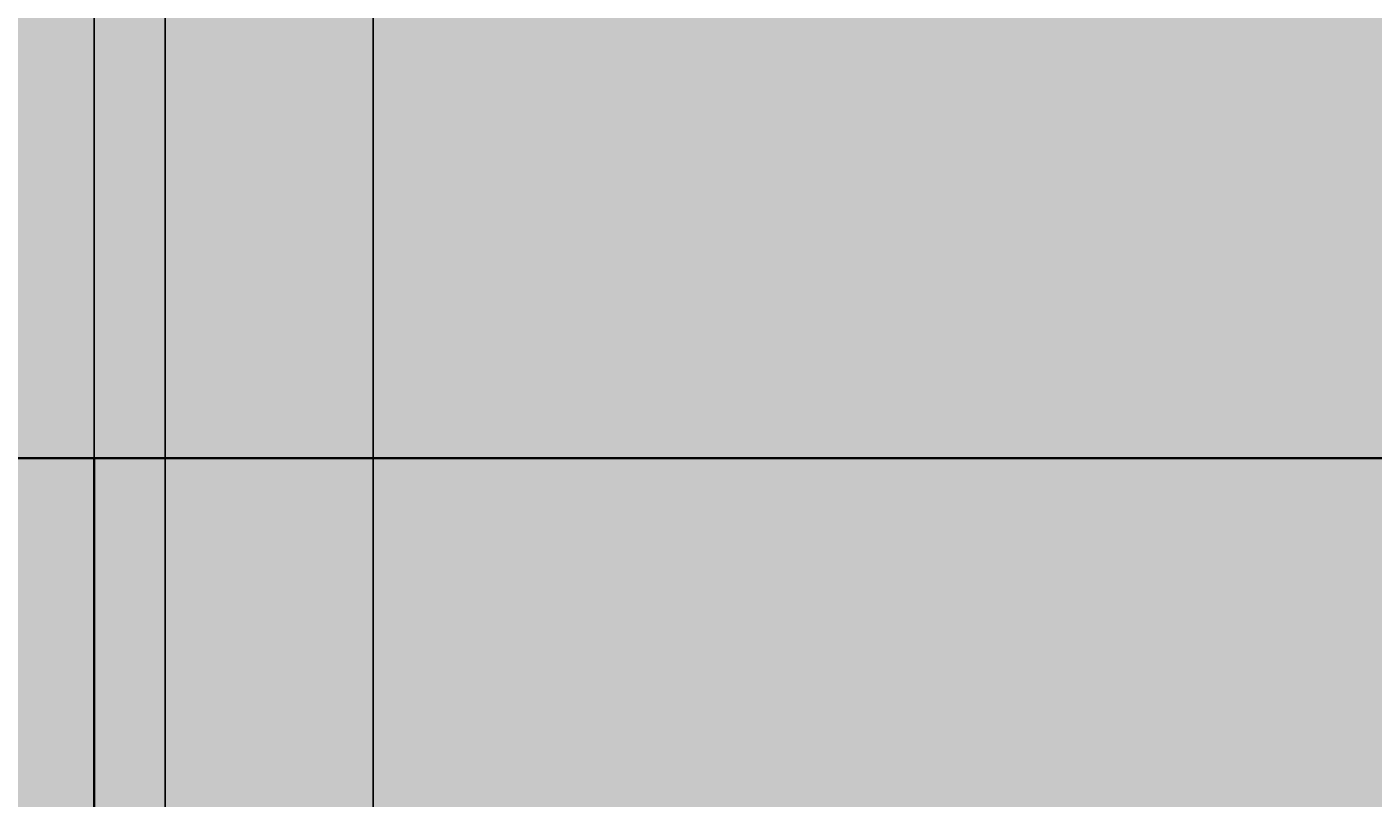
# Model space of a CAD drawing. Units: feet. Extents: x 2695 to 2912, y 795 to 1139.
# Tile 66 of 83: x 2769 to 2805, y 1041 to 1062. Entities that reach past the tile are written whole.
import ezdxf

# ---------------------------------------------------------------- set-up
doc = ezdxf.new("R2010")
doc.units = ezdxf.units.FT
for name, color, linetype, lineweight in [('A-ANNO-DIMS', 2, 'Continuous', 18), ('A-ELEV', 7, 'Continuous', 35), ('A-ELEV-PATT', 252, 'Continuous', 13)]:
    doc.layers.add(name, color=color, linetype=linetype, lineweight=lineweight)
doc.styles.get("Standard").update_dxf_attribs({"font": 'arial.ttf'})
doc.dimstyles.get("Standard").update_dxf_attribs({"dimtxt": 0.18, "dimasz": 0.18, "dimexe": 0.18, "dimexo": 0.0625, "dimgap": 0.09, "dimtad": 0, "dimtih": 1, "dimtoh": 1, "dimdec": 1, "dimzin": 0, "dimdsep": 46, "dimlunit": 3, "dimtxsty": 'Standard', "dimcen": 0.09, "dimadec": 0, "dimazin": 0, "dimtfac": 1, "dimtdec": 1, "dimtofl": 0, "dimtmove": 0, "dimatfit": 3, "dimfxl": 1, "dimtolj": 1, "dimtzin": 0, "dimarcsym": 0})

# ---------------------------------------------------------------- blocks, each defined once
blk = doc.blocks.new('*D8')
at = {"layer": 'A-ANNO-DIMS', "color": 0, "lineweight": -2, "transparency": 16777216}
for p, q in [((2715.885, 1050.373), (2715.885, 1138.886)), ((2716.065, 1138.706), (2742.866, 1138.706)), ((2770.456, 1138.706), (2743.655, 1138.706)), ((2770.636, 1122.993), (2770.636, 1138.886))]:
    blk.add_line(p, q, dxfattribs=at)
at = {"layer": 'A-ANNO-DIMS', "color": 0, "transparency": 16777216}
for points in [[(2716.065, 1138.736), (2716.065, 1138.676), (2715.885, 1138.706)], [(2770.456, 1138.736), (2770.456, 1138.676), (2770.636, 1138.706)]]:
    blk.add_solid(points, dxfattribs=at)
at = {"layer": 'Defpoints', "color": 0, "transparency": 16777216}
for p in [(2770.636, 1138.706), (2770.636, 1122.931), (2715.885, 1050.311)]:
    blk.add_point(p, dxfattribs=at)
at = {"layer": 'A-ANNO-DIMS', "color": 0, "transparency": 16777216, "insert": (2743.261, 1138.706), "char_height": 0.18, "attachment_point": 5}
blk.add_mtext('\\A1;54.75', dxfattribs=at)
blk = doc.blocks.new('*D9')
at = {"layer": 'A-ANNO-DIMS', "color": 0, "lineweight": -2, "transparency": 16777216}
for p, q in [((2770.636, 1122.993), (2770.636, 1138.886)), ((2770.816, 1138.706), (2773.942, 1138.706)), ((2777.854, 1138.706), (2774.728, 1138.706)), ((2778.034, 1020.886), (2778.034, 1138.886))]:
    blk.add_line(p, q, dxfattribs=at)
at = {"layer": 'A-ANNO-DIMS', "color": 0, "transparency": 16777216}
for points in [[(2770.816, 1138.736), (2770.816, 1138.676), (2770.636, 1138.706)], [(2777.854, 1138.736), (2777.854, 1138.676), (2778.034, 1138.706)]]:
    blk.add_solid(points, dxfattribs=at)
at = {"layer": 'Defpoints', "color": 0, "transparency": 16777216}
for p in [(2778.034, 1138.706), (2770.636, 1122.931), (2778.034, 1020.824)]:
    blk.add_point(p, dxfattribs=at)
at = {"layer": 'A-ANNO-DIMS', "color": 0, "transparency": 16777216, "insert": (2774.335, 1138.706), "char_height": 0.18, "attachment_point": 5}
blk.add_mtext('\\A1;7.398', dxfattribs=at)
blk = doc.blocks.new('*D10')
at = {"layer": 'A-ANNO-DIMS', "color": 0, "lineweight": -2, "transparency": 16777216}
for p, q in [((2778.034, 1020.886), (2778.034, 1138.886)), ((2778.214, 1138.706), (2810.411, 1138.706)), ((2843.395, 1138.706), (2811.198, 1138.706)), ((2843.575, 1020.886), (2843.575, 1138.886))]:
    blk.add_line(p, q, dxfattribs=at)
at = {"layer": 'A-ANNO-DIMS', "color": 0, "transparency": 16777216}
for points in [[(2778.214, 1138.736), (2778.214, 1138.676), (2778.034, 1138.706)], [(2843.395, 1138.736), (2843.395, 1138.676), (2843.575, 1138.706)]]:
    blk.add_solid(points, dxfattribs=at)
at = {"layer": 'Defpoints', "color": 0, "transparency": 16777216}
for p in [(2843.575, 1138.706), (2778.034, 1020.824), (2843.575, 1020.824)]:
    blk.add_point(p, dxfattribs=at)
at = {"layer": 'A-ANNO-DIMS', "color": 0, "transparency": 16777216, "insert": (2810.805, 1138.706), "char_height": 0.18, "attachment_point": 5}
blk.add_mtext('\\A1;65.54', dxfattribs=at)
blk = doc.blocks.new('*D48')
at = {"layer": 'A-ANNO-DIMS', "color": 0, "lineweight": -2, "transparency": 16777216}
for p, q in [((2770.636, 972.03), (2770.636, 1138.886)), ((2770.816, 1138.706), (2771.263, 1138.706)), ((2772.342, 1138.706), (2771.894, 1138.706)), ((2772.522, 972.03), (2772.522, 1138.886))]:
    blk.add_line(p, q, dxfattribs=at)
at = {"layer": 'A-ANNO-DIMS', "color": 0, "transparency": 16777216}
for points in [[(2770.816, 1138.736), (2770.816, 1138.676), (2770.636, 1138.706)], [(2772.342, 1138.736), (2772.342, 1138.676), (2772.522, 1138.706)]]:
    blk.add_solid(points, dxfattribs=at)
at = {"layer": 'Defpoints', "color": 0, "transparency": 16777216}
for p in [(2772.522, 1138.706), (2770.636, 971.967), (2772.522, 971.967)]:
    blk.add_point(p, dxfattribs=at)
at = {"layer": 'A-ANNO-DIMS', "color": 0, "transparency": 16777216, "insert": (2771.579, 1138.706), "char_height": 0.18, "attachment_point": 5}
blk.add_mtext('\\A1;1.89', dxfattribs=at)
blk = doc.blocks.new('*D49')
at = {"layer": 'A-ANNO-DIMS', "color": 0, "lineweight": -2, "transparency": 16777216}
for p, q in [((2772.522, 972.03), (2772.522, 1138.886)), ((2772.702, 1138.706), (2790.888, 1138.706)), ((2809.861, 1138.706), (2791.674, 1138.706)), ((2810.041, 972.03), (2810.041, 1138.886))]:
    blk.add_line(p, q, dxfattribs=at)
at = {"layer": 'A-ANNO-DIMS', "color": 0, "transparency": 16777216}
for points in [[(2772.702, 1138.736), (2772.702, 1138.676), (2772.522, 1138.706)], [(2809.861, 1138.736), (2809.861, 1138.676), (2810.041, 1138.706)]]:
    blk.add_solid(points, dxfattribs=at)
at = {"layer": 'Defpoints', "color": 0, "transparency": 16777216}
for p in [(2810.041, 1138.706), (2772.522, 971.967), (2810.041, 971.967)]:
    blk.add_point(p, dxfattribs=at)
at = {"layer": 'A-ANNO-DIMS', "color": 0, "transparency": 16777216, "insert": (2791.281, 1138.706), "char_height": 0.18, "attachment_point": 5}
blk.add_mtext('\\A1;37.52', dxfattribs=at)

msp = doc.modelspace()

# ---------------------------------------------------------------- hatches: boundary and pattern name
at = {"layer": 'A-ELEV-PATT'}
h = msp.add_hatch(color=256, dxfattribs=at)
h.set_gradient(color1=(255, 255, 255), tint=1)
h.paths.add_polyline_path([(2770.6361, 1122.9306), (2710.6361, 1122.9306), (2710.6361, 1118.4096), (2770.6361, 1118.4096)])
h.paths.add_polyline_path([(2890.6361, 1107.8588), (2770.6361, 1107.8588), (2770.6361, 1103.3378), (2890.6361, 1103.3378)])
h.paths.add_polyline_path([(2890.6361, 1062.9306), (2710.6361, 1062.9306), (2710.6361, 1056.9306), (2710.6361, 936.9306), (2710.6361, 924.3105), (2716.5358, 924.3105), (2890.6361, 924.3105), (2890.6361, 936.9306), (2715.8852, 936.9306), (2715.8852, 1050.3105), (2890.6361, 1050.3105)])
h.paths.add_polyline_path([(2716.5358, 924.3105), (2710.6361, 924.3105), (2710.6361, 810.9306), (2716.5358, 810.9306)])
h = msp.add_hatch(color=256, dxfattribs=at)
h.set_gradient(color1=(147, 149, 152), color2=(147, 149, 152), tint=1)
h.paths.add_polyline_path([(2770.6361, 1118.4096), (2710.6361, 1118.4096), (2710.6361, 1062.9306), (2770.6361, 1062.9306)])
h.paths.add_polyline_path([(2890.6361, 1103.3378), (2770.6361, 1103.3378), (2770.6361, 1062.9306), (2890.6361, 1062.9306)])
h.paths.add_polyline_path([(2730.7081, 1048.1052), (2755.1125, 1048.1052), (2755.1125, 936.9306), (2770.6361, 936.9306), (2770.6361, 1050.3105), (2715.8852, 1050.3105), (2715.8852, 936.9306), (2730.7081, 936.9306)])
h.paths.add_polyline_path([(2890.6361, 1050.3105), (2770.6361, 1050.3105), (2770.6361, 971.9673), (2778.0341, 971.9673), (2778.0341, 1020.8235), (2843.575, 1020.8235), (2843.575, 971.9673), (2890.6361, 971.9673)])
h.paths.add_polyline_path([(2888.1882, 970.7156), (2843.575, 970.7156), (2843.575, 964.8267), (2888.1882, 964.8267)])
h.paths.add_polyline_path([(2888.1882, 964.1328), (2843.575, 964.1328), (2843.575, 956.614), (2888.1882, 956.614)])
h.paths.add_polyline_path([(2888.1882, 955.9202), (2843.575, 955.9202), (2843.575, 949.2892), (2888.1882, 949.2892)])
h.paths.add_polyline_path([(2888.1882, 948.5954), (2843.575, 948.5954), (2843.575, 941.3507), (2888.1882, 941.3507)])
h.paths.add_polyline_path([(2888.1882, 940.6569), (2843.575, 940.6569), (2843.575, 936.9306), (2888.1882, 936.9306)])
h.paths.add_polyline_path([(2890.6361, 970.7156), (2888.9368, 970.7156), (2888.9368, 964.8267), (2890.6361, 964.8267)])
h.paths.add_polyline_path([(2890.6361, 964.1328), (2888.9368, 964.1328), (2888.9368, 956.614), (2890.6361, 956.614)])
h.paths.add_polyline_path([(2890.6361, 955.9202), (2888.9368, 955.9202), (2888.9368, 949.2892), (2890.6361, 949.2892)])
h.paths.add_polyline_path([(2890.6361, 940.6569), (2888.9368, 940.6569), (2888.9368, 936.9306), (2890.6361, 936.9306)])
h.paths.add_polyline_path([(2890.6361, 948.5954), (2888.9368, 948.5954), (2888.9368, 941.3507), (2890.6361, 941.3507)])
h.paths.add_polyline_path([(2772.5216, 970.7156), (2770.6361, 970.7156), (2770.6361, 964.8267), (2772.5216, 964.8267)])
h.paths.add_polyline_path([(2772.5216, 964.1328), (2770.6361, 964.1328), (2770.6361, 956.614), (2772.5216, 956.614)])
h.paths.add_polyline_path([(2772.5216, 955.9202), (2770.6361, 955.9202), (2770.6361, 949.2892), (2772.5216, 949.2892)])
h.paths.add_polyline_path([(2772.5216, 948.5954), (2770.6361, 948.5954), (2770.6361, 941.3507), (2772.5216, 941.3507)])
h.paths.add_polyline_path([(2772.5216, 940.6569), (2770.6361, 940.6569), (2770.6361, 936.9306), (2772.5216, 936.9306)])
h.paths.add_polyline_path([(2778.0341, 940.6569), (2773.2702, 940.6569), (2773.2702, 936.9306), (2778.0341, 936.9306)])
h.paths.add_polyline_path([(2778.0341, 970.7156), (2773.2702, 970.7156), (2773.2702, 964.8267), (2778.0341, 964.8267)])
h.paths.add_polyline_path([(2778.0341, 964.1328), (2773.2702, 964.1328), (2773.2702, 956.614), (2778.0341, 956.614)])
h.paths.add_polyline_path([(2778.0341, 955.9202), (2773.2702, 955.9202), (2773.2702, 949.2892), (2778.0341, 949.2892)])
h.paths.add_polyline_path([(2778.0341, 948.5954), (2773.2702, 948.5954), (2773.2702, 941.3507), (2778.0341, 941.3507)])
h.paths.add_polyline_path([(2810.0407, 940.6569), (2780.0341, 940.6569), (2780.0341, 936.9306), (2810.0407, 936.9306)])
h.paths.add_polyline_path([(2890.6361, 924.3105), (2770.6361, 924.3105), (2770.6361, 810.9306), (2773.5029, 810.9306), (2773.5029, 905.5143), (2805.9398, 905.5143), (2838.3767, 905.5143), (2838.3767, 810.9306), (2890.6361, 810.9306)])

# ---------------------------------------------------------------- linework, layer by layer
at = {"layer": 'A-ELEV'}
for p, q in [((2890.6361, 1050.3105), (2715.8852, 1050.3105)), ((2770.6361, 1050.3105), (2770.6361, 936.9306))]:
    msp.add_line(p, q, dxfattribs=at)
msp.add_lwpolyline([(2890.6361, 1050.3105), (2715.8852, 1050.3105)], dxfattribs=at)

# ---------------------------------------------------------------- dimensions: what is measured, and where the dimension line sits
at = {"layer": 'A-ANNO-DIMS'}
for base, p1, p2, override, picture, middle in [((2770.6361, 1138.7056), (2715.8852, 1050.3105), (2770.6361, 1122.9306), {"dimdec": 2, "dimlfac": 1, "dimrnd": 0, "dimzin": 0, "dimdsep": 46, "dimlunit": 2}, '*D8', (2743.2606, 1138.7056)), ((2778.0341, 1138.7056), (2770.6361, 1122.9306), (2778.0341, 1020.8235), {"dimdec": 3, "dimlfac": 1, "dimrnd": 0, "dimzin": 0, "dimdsep": 46, "dimlunit": 2}, '*D9', (2774.3351, 1138.7056)), ((2772.5216, 1138.7056), (2770.6361, 971.9673), (2772.5216, 971.9673), {"dimdec": 2, "dimlfac": 1, "dimrnd": 0, "dimzin": 0, "dimdsep": 46, "dimlunit": 2}, '*D48', (2771.5788, 1138.7056)), ((2810.0407, 1138.7056), (2772.5216, 971.9673), (2810.0407, 971.9673), {"dimdec": 2, "dimlfac": 1, "dimrnd": 0, "dimzin": 0, "dimdsep": 46, "dimlunit": 2}, '*D49', (2791.2811, 1138.7056)), ((2843.575, 1138.7056), (2778.0341, 1020.8235), (2843.575, 1020.8235), {"dimdec": 2, "dimlfac": 1, "dimrnd": 0, "dimzin": 0, "dimdsep": 46, "dimlunit": 2}, '*D10', (2810.8045, 1138.7056))]:
    dim = msp.add_linear_dim(base=base, p1=p1, p2=p2, dimstyle='Standard', override=override, dxfattribs=at)
    dim.commit()
    dim.dimension.update_dxf_attribs({"geometry": picture, "text_midpoint": middle})

doc.saveas('drawing.dxf')
